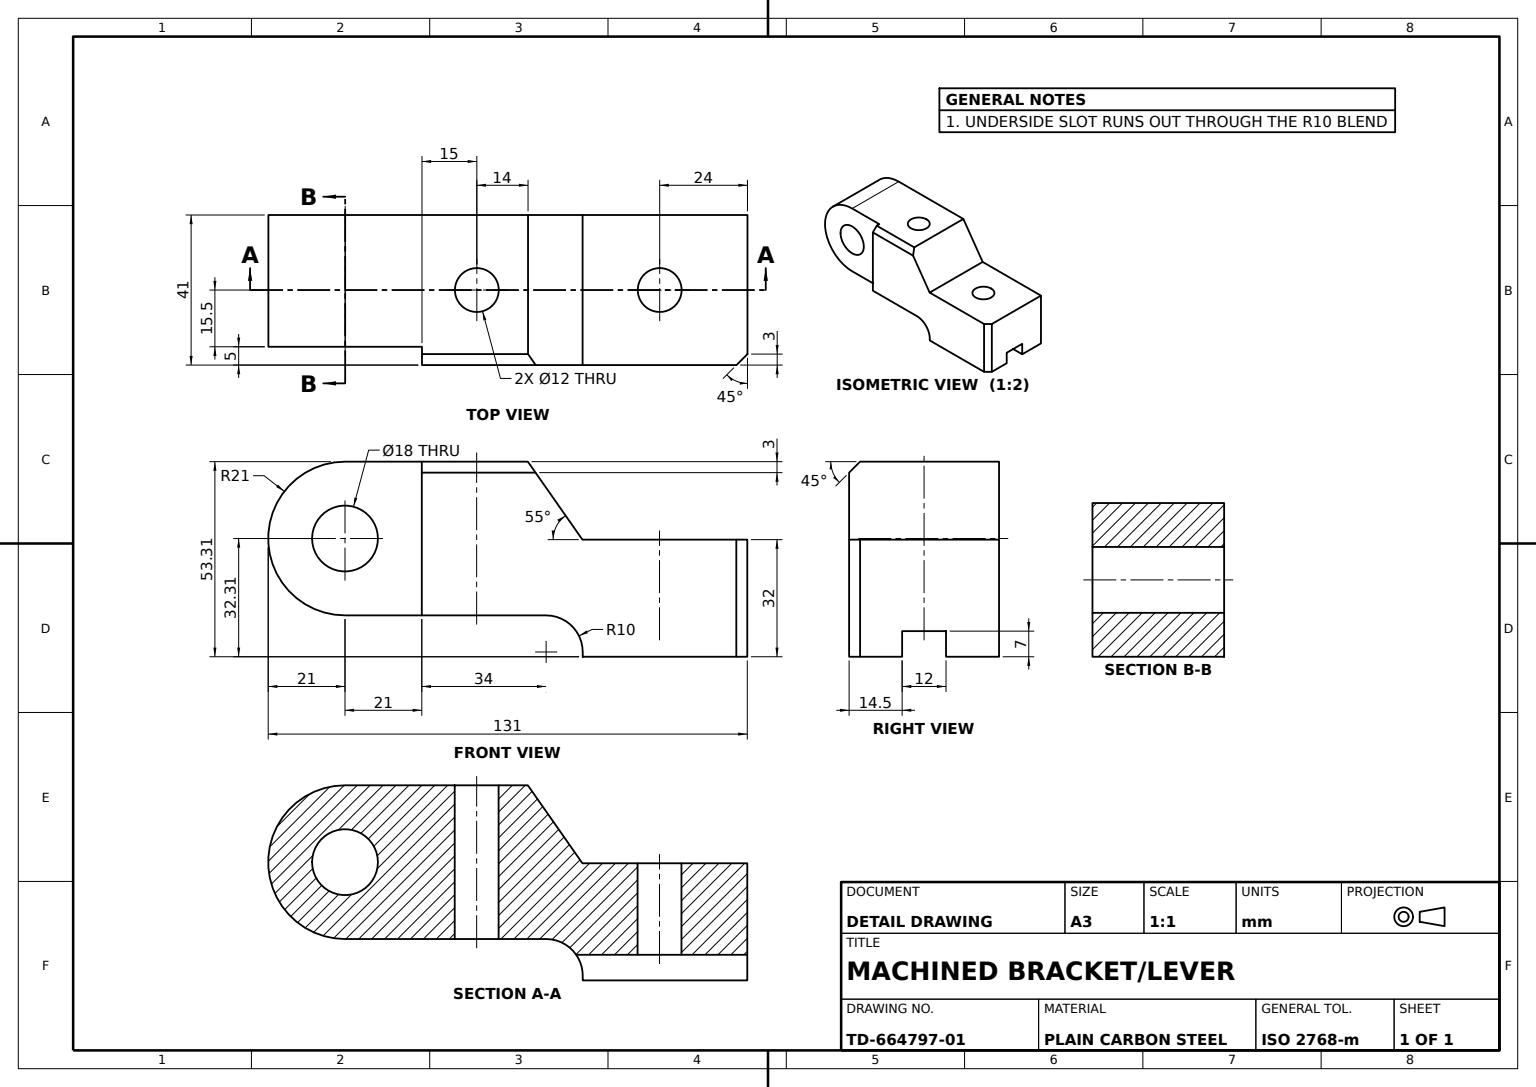
from build123d import *

# Parameters (mm, degrees)
LEVER_BODY_41MM_DEPTH     = 20.5
PIVOT_EYE_BOSS_DEPTH      = 15.5
PIVOT_EYE_BOSS_DEPTH_BACK = 20.5
SKETCH1_4_R               = 9
EDGE_CHAMFER_3X45_A_SIZE  = 3
EDGE_CHAMFER_3X45_B_SIZE  = 3
UNDERSIDE_SLOT_SKETCH_W   = 12
UNDERSIDE_SLOT_SKETCH_H   = 7
UNDERSIDE_SLOT_DEPTH      = 145.5
TOP_HOLES_SKETCH_R        = 6
TOP_HOLES_2X_DEPTH        = 155.5


with BuildPart() as part:
    # Lever Profile Sketch → Lever Body 41mm (new, symmetric)
    with BuildSketch(Plane.XY):
        with BuildLine():
            Line((50, 21), (21, 21))
            Line((21, 21), (21, -21))
            Line((21, -21), (55, -21))
            ThreePointArc((55, -21), (62.071067812, -23.928932188), (65, -31))
            Line((65, -31), (65, -32.305162606))
            Line((65, -32.305162606), (110, -32.305162606))
            Line((110, -32.305162606), (110, -0.305162606))
            Line((110, -0.305162606), (64.918035459, -0.305162606))
            Line((64.918035459, -0.305162606), (50, 21))
        make_face()
    extrude(amount=LEVER_BODY_41MM_DEPTH, both=True)

    # Sketch1_4 → Pivot Eye Boss (add, two sides: drawn at the far end of the back side and taken through both)
    with BuildSketch(Plane.XY.offset(-PIVOT_EYE_BOSS_DEPTH_BACK)):
        with BuildLine():
            Line((21, 21), (0, 21))
            ThreePointArc((0, 21), (-21, 0), (0, -21))
            Line((0, -21), (21, -21))
            Line((21, -21), (21, 21))
        make_face()
        Circle(SKETCH1_4_R, mode=Mode.SUBTRACT)
    extrude(amount=PIVOT_EYE_BOSS_DEPTH + PIVOT_EYE_BOSS_DEPTH_BACK)

    # Edge Chamfer 3x45 A
    edge_chamfer_3x45_a_edges = [part.edges().sort_by_distance(p)[0] for p in [
        (35.5, 21, 20.5),
    ]]
    chamfer(edge_chamfer_3x45_a_edges, length=EDGE_CHAMFER_3X45_A_SIZE)

    # Edge Chamfer 3x45 B
    edge_chamfer_3x45_b_edges = [part.edges().sort_by_distance(p)[0] for p in [
        (110, -16.305162606, 20.5),
    ]]
    chamfer(edge_chamfer_3x45_b_edges, length=EDGE_CHAMFER_3X45_B_SIZE)

    # Underside Slot Sketch → Underside Slot (cut)
    with BuildSketch(Plane(origin=(110, 0, 0), x_dir=(0, 0, -1), z_dir=(1, 0, 0))):
        with Locations((0, -28.805162606)):
            Rectangle(UNDERSIDE_SLOT_SKETCH_W, UNDERSIDE_SLOT_SKETCH_H)
    extrude(amount=-UNDERSIDE_SLOT_DEPTH, mode=Mode.SUBTRACT)

    # Top Holes Sketch → Top Holes 2x (cut)
    with BuildSketch(Plane(origin=(0, 21, 0), x_dir=(1, 0, 0), z_dir=(0, 1, 0))):
        with Locations(Location((36, 0, 0), (0, 0, 270))):
            Circle(TOP_HOLES_SKETCH_R)
        with Locations(Location((86, 0, 0), (0, 0, 270))):
            Circle(TOP_HOLES_SKETCH_R)
    extrude(amount=-TOP_HOLES_2X_DEPTH, mode=Mode.SUBTRACT)


solid = part.part
